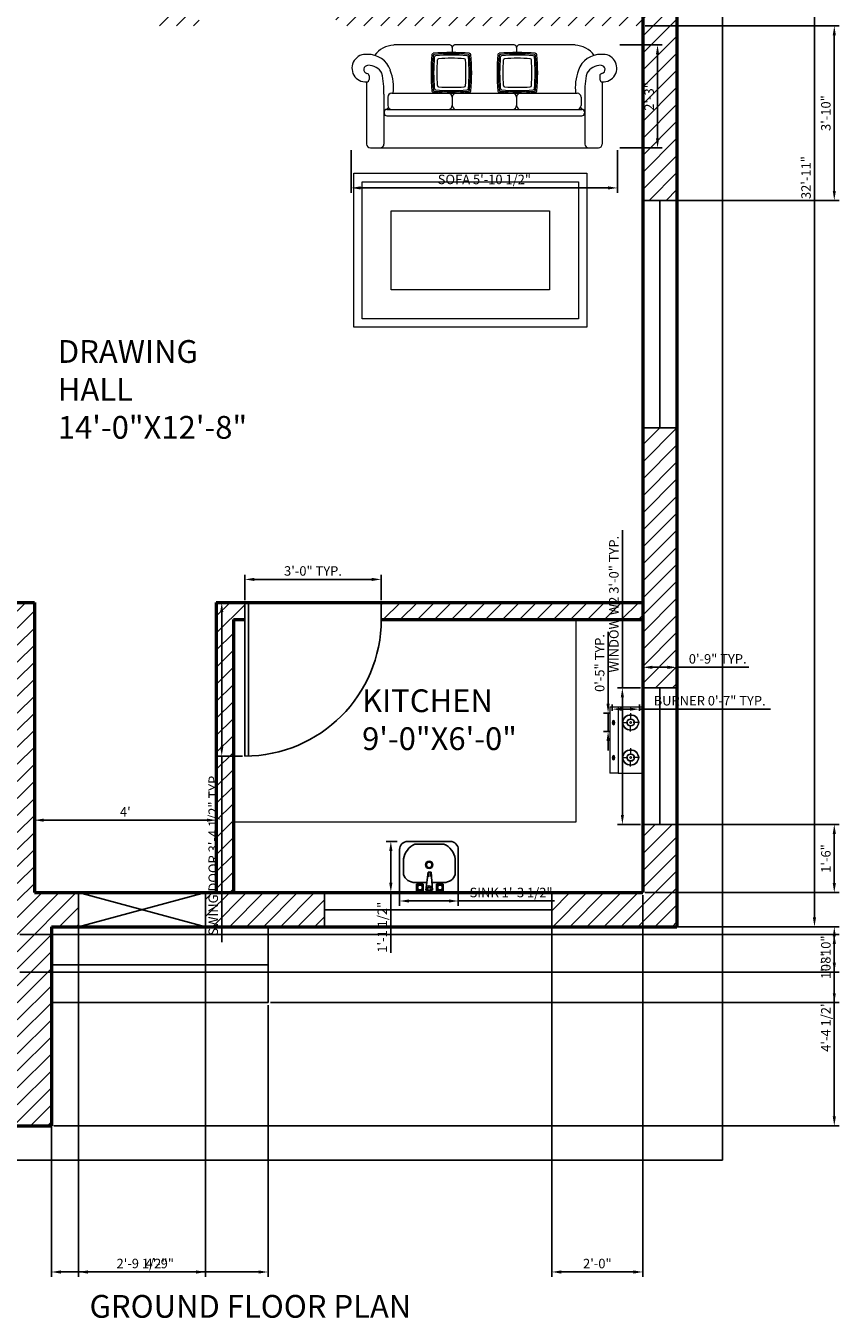
# Model space of a CAD drawing. Units: inches. Extents: x 3542 to 3908, y 2103 to 2666.
# Tile 2 of 4: x 3693 to 3908, y 2103 to 2444. Entities that reach past the tile are written whole.
import ezdxf

# ---------------------------------------------------------------- set-up
doc = ezdxf.new("R2010")
doc.units = ezdxf.units.IN
for name, color, linetype, lineweight in [('A-ANNO-DIMS', 2, 'Continuous', 18), ('A-ANNO-TEXT', 7, 'Continuous', 25), ('A-AREA-IDEN', 7, 'Continuous', 25), ('A-DOOR', 3, 'Continuous', 25), ('A-EQPM', 8, 'Continuous', 18), ('A-FLOR-CASE', 8, 'Continuous', 18), ('A-FLOR-FIXT', 9, 'Continuous', 25), ('A-FLOR-STRS', 7, 'Continuous', 25), ('A-FURN', 8, 'Continuous', 18), ('A-GLAZ', 5, 'Continuous', 25), ('A-WALL', 7, 'Continuous', 50), ('A-WALL-PATT', 252, 'Continuous', 13), ('C-PROP', 7, 'Continuous', 25)]:
    doc.layers.add(name, color=color, linetype=linetype, lineweight=lineweight)
doc.styles.get("Standard").update_dxf_attribs({"font": 'arial.ttf'})
doc.dimstyles.new('ISO-25', dxfattribs={"dimtxt": 2.5, "dimasz": 2.5, "dimexe": 1.25, "dimexo": 0.625, "dimtad": 1, "dimdec": 0, "dimlunit": 3, "dimtxsty": 'Standard', "dimcen": 2.5, "dimadec": 0, "dimazin": 0, "dimtfac": 1, "dimtdec": 0, "dimtmove": 0, "dimatfit": 3, "dimfxl": 1, "dimarcsym": 0})

# ---------------------------------------------------------------- blocks, each defined once
blk = doc.blocks.new('*D1')
at = {"layer": 'A-ANNO-DIMS', "color": 0, "lineweight": -2, "transparency": 16777216}
for p, q in [((3695.14, 2225.85), (3695.14, 2235.83)), ((3743.14, 2225.85), (3743.14, 2235.83)), ((3740.64, 2234.58), (3697.64, 2234.58))]:
    blk.add_line(p, q, dxfattribs=at)
at = {"layer": 'A-ANNO-DIMS', "color": 0, "transparency": 16777216}
for points in [[(3697.64, 2235), (3697.64, 2234.17), (3695.14, 2234.58)], [(3740.64, 2235), (3740.64, 2234.17), (3743.14, 2234.58)]]:
    blk.add_solid(points, dxfattribs=at)
at = {"layer": 'Defpoints', "color": 0, "transparency": 16777216}
for p in [(3695.14, 2234.58), (3695.14, 2225.23), (3743.14, 2225.23)]:
    blk.add_point(p, dxfattribs=at)
at = {"layer": 'A-ANNO-DIMS', "color": 0, "transparency": 16777216, "insert": (3719.14, 2236.46), "char_height": 2.5, "attachment_point": 5}
blk.add_mtext("4'", dxfattribs=at)
blk = doc.blocks.new('*D11')
at = {"layer": 'A-ANNO-DIMS', "color": 0, "lineweight": -2, "transparency": 16777216}
for p, q in [((3877.27, 2601.48), (3902.16, 2601.48)), ((3900.91, 2208.98), (3900.91, 2598.98)), ((3877.27, 2206.48), (3902.16, 2206.48))]:
    blk.add_line(p, q, dxfattribs=at)
at = {"layer": 'A-ANNO-DIMS', "color": 0, "transparency": 16777216}
for points in [[(3900.5, 2598.98), (3901.33, 2598.98), (3900.91, 2601.48)], [(3900.5, 2208.98), (3901.33, 2208.98), (3900.91, 2206.48)]]:
    blk.add_solid(points, dxfattribs=at)
at = {"layer": 'Defpoints', "color": 0, "transparency": 16777216}
for p in [(3876.64, 2601.48), (3900.91, 2601.48), (3876.64, 2206.48)]:
    blk.add_point(p, dxfattribs=at)
at = {"layer": 'A-ANNO-DIMS', "color": 0, "transparency": 16777216, "insert": (3899.01, 2403.98), "char_height": 2.5, "attachment_point": 5, "rotation": 90}
blk.add_mtext('32\'-11"', dxfattribs=at)
blk = doc.blocks.new('A$C796C3687')
for p, q in [((760, 800), (324, 800)), ((760, 800), (324, 800)), ((779, 780), (779, 742)), ((779, 780), (779, 742)), ((1260, 800), (797, 800)), ((1260, 800), (797, 800)), ((1279, 780), (1279, 742)), ((1279, 780), (1279, 742)), ((1734, 800), (1297, 800)), ((1734, 800), (1297, 800)), ((113, 513), (113, 30)), ((113, 513), (113, 30)), ((132, 560), (132, 533)), ((132, 560), (132, 533)), ((1926, 560), (1926, 533)), ((1926, 560), (1926, 533)), ((1945, 513), (1945, 30)), ((1945, 513), (1945, 30)), ((248, 418), (248, 30)), ((248, 418), (248, 30)), ((308, 425), (749, 425)), ((308, 425), (749, 425)), ((809, 425), (1249, 425)), ((809, 425), (1249, 425)), ((1309, 425), (1750, 425)), ((1309, 425), (1750, 425)), ((1810, 418), (1810, 30)), ((1810, 418), (1810, 30)), ((278, 395), (278, 330)), ((278, 395), (278, 330)), ((779, 395), (779, 330)), ((779, 395), (779, 330)), ((1279, 395), (1279, 330)), ((1279, 395), (1279, 330)), ((1780, 395), (1780, 330)), ((1780, 395), (1780, 330)), ((250, 280), (250, 270)), ((250, 280), (250, 270)), ((270, 300), (1787, 300)), ((270, 300), (1787, 300)), ((270, 250), (1787, 250)), ((270, 250), (1787, 250)), ((1807, 280), (1807, 270)), ((1807, 280), (1807, 270)), ((143, 0), (1915, 0)), ((143, 0), (1915, 0))]:
    blk.add_line(p, q)
for centre, radius, start, end in [((106, 620), 107, 83.1024, 273.7108), ((106, 620), 107, 83.1024, 273.7108), ((128, 547), 179, 18.5515, 93.0451), ((128, 547), 179, 18.5515, 93.0451), ((338, 593), 207, 94.0017, 142.3205), ((338, 593), 207, 94.0017, 142.3205), ((2093, 584), 1479, 174.4972, 185.5028), ((2093, 584), 1479, 174.4972, 185.5028), ((631, 725), 10, 95.5028, 174.4972), ((631, 725), 10, 95.5028, 174.4972), ((2093, 584), 1469, 174.8217, 185.1783), ((2093, 584), 1469, 174.8217, 185.1783), ((772, -737), 1479, 84.4972, 95.5028), ((772, -737), 1479, 84.4972, 95.5028), ((640, 716), 10, 95.1783, 174.8217), ((640, 716), 10, 95.1783, 174.8217), ((2093, 584), 1459, 175.1522, 184.8478), ((2093, 584), 1459, 175.1522, 184.8478), ((772, -737), 1469, 84.8217, 95.1783), ((772, -737), 1469, 84.8217, 95.1783), ((650, 706), 10, 94.8478, 175.1522), ((650, 706), 10, 94.8478, 175.1522), ((772, -737), 1459, 85.1522, 94.8478), ((772, -737), 1459, 85.1522, 94.8478), ((759, 780), 20, 0, 94.3856), ((759, 780), 20, 0, 94.3856), ((799, 780), 20, 85.6144, 180), ((799, 780), 20, 85.6144, 180), ((895, 706), 10, 4.8478, 85.1522), ((895, 706), 10, 4.8478, 85.1522), ((904, 716), 10, 5.1783, 84.8217), ((904, 716), 10, 5.1783, 84.8217), ((-549, 584), 1459, 355.1522, 4.8478), ((-549, 584), 1459, 355.1522, 4.8478), ((913, 725), 10, 5.5028, 84.4972), ((913, 725), 10, 5.5028, 84.4972), ((-549, 584), 1469, 354.8217, 5.1783), ((-549, 584), 1469, 354.8217, 5.1783), ((-549, 584), 1479, 354.4972, 5.5028), ((-549, 584), 1479, 354.4972, 5.5028), ((2606, 584), 1479, 174.4972, 185.5028), ((2606, 584), 1479, 174.4972, 185.5028), ((1144, 725), 10, 95.5028, 174.4972), ((1144, 725), 10, 95.5028, 174.4972), ((2606, 584), 1469, 174.8217, 185.1783), ((2606, 584), 1469, 174.8217, 185.1783), ((1285, -737), 1479, 84.4972, 95.5028), ((1285, -737), 1479, 84.4972, 95.5028), ((1154, 716), 10, 95.1783, 174.8217), ((1154, 716), 10, 95.1783, 174.8217), ((2606, 584), 1459, 175.1522, 184.8478), ((2606, 584), 1459, 175.1522, 184.8478), ((1285, -737), 1469, 84.8217, 95.1783), ((1285, -737), 1469, 84.8217, 95.1783), ((1163, 706), 10, 94.8478, 175.1522), ((1163, 706), 10, 94.8478, 175.1522), ((1285, -737), 1459, 85.1522, 94.8478), ((1285, -737), 1459, 85.1522, 94.8478), ((1259, 780), 20, 0, 94.3856), ((1259, 780), 20, 0, 94.3856), ((1299, 780), 20, 85.6144, 180), ((1299, 780), 20, 85.6144, 180), ((1408, 706), 10, 4.8478, 85.1522), ((1408, 706), 10, 4.8478, 85.1522), ((1417, 716), 10, 5.1783, 84.8217), ((1417, 716), 10, 5.1783, 84.8217), ((-36, 584), 1459, 355.1522, 4.8478), ((-36, 584), 1459, 355.1522, 4.8478), ((1426, 725), 10, 5.5028, 84.4972), ((1426, 725), 10, 5.5028, 84.4972), ((-36, 584), 1469, 354.8217, 5.1783), ((-36, 584), 1469, 354.8217, 5.1783), ((-36, 584), 1479, 354.4972, 5.5028), ((-36, 584), 1479, 354.4972, 5.5028), ((1719, 593), 207, 37.6795, 85.9983), ((1719, 593), 207, 37.6795, 85.9983), ((1929, 547), 179, 86.9549, 161.4485), ((1929, 547), 179, 86.9549, 161.4485), ((1951, 620), 107, 266.2892, 96.8976), ((1951, 620), 107, 266.2892, 96.8976), ((122, 610), 31.2, 88.5716, 258.3882), ((122, 610), 31.2, 88.5716, 258.3882), ((126, 520), 122, 29.5431, 91.582), ((126, 520), 122, 29.5431, 91.582), ((-50, 470), 372, 353.0593, 21.0381), ((-50, 470), 372, 353.0593, 21.0381), ((2093, 584), 1434, 176.0063, 183.9937), ((2093, 584), 1434, 176.0063, 183.9937), ((673, 683), 10, 93.9937, 176.0063), ((673, 683), 10, 93.9937, 176.0063), ((772, -737), 1434, 86.0063, 93.9937), ((772, -737), 1434, 86.0063, 93.9937), ((871, 683), 10, 3.9937, 86.0063), ((871, 683), 10, 3.9937, 86.0063), ((-549, 584), 1434, 356.0063, 3.9937), ((-549, 584), 1434, 356.0063, 3.9937), ((2606, 584), 1434, 176.0063, 183.9937), ((2606, 584), 1434, 176.0063, 183.9937), ((1186, 683), 10, 93.9937, 176.0063), ((1186, 683), 10, 93.9937, 176.0063), ((1285, -737), 1434, 86.0063, 93.9937), ((1285, -737), 1434, 86.0063, 93.9937), ((1384, 683), 10, 3.9937, 86.0063), ((1384, 683), 10, 3.9937, 86.0063), ((-36, 584), 1434, 356.0063, 3.9937), ((-36, 584), 1434, 356.0063, 3.9937), ((2107, 470), 372, 158.9619, 187.3268), ((2107, 470), 372, 158.9619, 187.3268), ((1932, 520), 122, 88.418, 150.4569), ((1932, 520), 122, 88.418, 150.4569), ((1936, 610), 31.2, 281.6118, 91.4284), ((1936, 610), 31.2, 281.6118, 91.4284), ((112, 533), 20, 273.7108, 0), ((112, 533), 20, 273.7108, 0), ((112, 560), 20, 0, 78.8393), ((112, 560), 20, 0, 78.8393), ((-351, 440), 599, 357.8297, 13.4516), ((-351, 440), 599, 357.8297, 13.4516), ((2408, 440), 599, 166.5484, 182.1703), ((2408, 440), 599, 166.5484, 182.1703), ((1946, 560), 20, 101.1607, 180), ((1946, 560), 20, 101.1607, 180), ((1946, 533), 20, 180, 266.2892), ((1946, 533), 20, 180, 266.2892), ((308, 395), 30, 90, 180), ((308, 395), 30, 90, 180), ((631, 443), 10, 185.5028, 264.4972), ((631, 443), 10, 185.5028, 264.4972), ((772, 1905), 1479, 264.4972, 275.5028), ((772, 1905), 1479, 264.4972, 275.5028), ((640, 452), 10, 185.1783, 264.8217), ((640, 452), 10, 185.1783, 264.8217), ((650, 462), 10, 184.8478, 265.1522), ((650, 462), 10, 184.8478, 265.1522), ((772, 1905), 1469, 264.8217, 275.1783), ((772, 1905), 1469, 264.8217, 275.1783), ((772, 1905), 1459, 265.1522, 274.8478), ((772, 1905), 1459, 265.1522, 274.8478), ((673, 485), 10, 183.9937, 266.0063), ((673, 485), 10, 183.9937, 266.0063), ((772, 1905), 1434, 266.0063, 273.9937), ((772, 1905), 1434, 266.0063, 273.9937), ((749, 395), 30, 0, 90), ((749, 395), 30, 0, 90), ((809, 395), 30, 90, 180), ((809, 395), 30, 90, 180), ((871, 485), 10, 273.9937, 356.0063), ((871, 485), 10, 273.9937, 356.0063), ((895, 462), 10, 274.8478, 355.1522), ((895, 462), 10, 274.8478, 355.1522), ((904, 452), 10, 275.1783, 354.8217), ((904, 452), 10, 275.1783, 354.8217), ((913, 443), 10, 275.5028, 354.4972), ((913, 443), 10, 275.5028, 354.4972), ((1144, 443), 10, 185.5028, 264.4972), ((1144, 443), 10, 185.5028, 264.4972), ((1285, 1905), 1479, 264.4972, 275.5028), ((1285, 1905), 1479, 264.4972, 275.5028), ((1154, 452), 10, 185.1783, 264.8217), ((1154, 452), 10, 185.1783, 264.8217), ((1163, 462), 10, 184.8478, 265.1522), ((1163, 462), 10, 184.8478, 265.1522), ((1285, 1905), 1469, 264.8217, 275.1783), ((1285, 1905), 1469, 264.8217, 275.1783), ((1285, 1905), 1459, 265.1522, 274.8478), ((1285, 1905), 1459, 265.1522, 274.8478), ((1186, 485), 10, 183.9937, 266.0063), ((1186, 485), 10, 183.9937, 266.0063), ((1285, 1905), 1434, 266.0063, 273.9937), ((1285, 1905), 1434, 266.0063, 273.9937), ((1249, 395), 30, 0, 90), ((1249, 395), 30, 0, 90), ((1309, 395), 30, 90, 180), ((1309, 395), 30, 90, 180), ((1384, 485), 10, 273.9937, 356.0063), ((1384, 485), 10, 273.9937, 356.0063), ((1408, 462), 10, 274.8478, 355.1522), ((1408, 462), 10, 274.8478, 355.1522), ((1417, 452), 10, 275.1783, 354.8217), ((1417, 452), 10, 275.1783, 354.8217), ((1426, 443), 10, 275.5028, 354.4972), ((1426, 443), 10, 275.5028, 354.4972), ((1750, 395), 30, 0, 90), ((1750, 395), 30, 0, 90), ((245, 338), 43.6, 273.0261, 327.6403), ((245, 338), 43.6, 273.0261, 327.6403), ((308, 330), 30, 180, 270), ((308, 330), 30, 180, 270), ((749, 330), 30, 270, 0), ((749, 330), 30, 270, 0), ((809, 330), 30, 180, 270), ((809, 330), 30, 180, 270), ((1249, 330), 30, 270, 0), ((1249, 330), 30, 270, 0), ((1309, 330), 30, 180, 270), ((1309, 330), 30, 180, 270), ((1750, 330), 30, 270, 0), ((1750, 330), 30, 270, 0), ((1812, 338), 43.6, 212.3597, 266.9739), ((1812, 338), 43.6, 212.3597, 266.9739), ((270, 280), 20, 90, 180), ((270, 280), 20, 90, 180), ((270, 270), 20, 180, 270), ((270, 270), 20, 180, 270), ((1787, 280), 20, 0, 90), ((1787, 280), 20, 0, 90), ((1787, 270), 20, 270, 0), ((1787, 270), 20, 270, 0), ((143, 30), 30, 180, 270), ((143, 30), 30, 180, 270), ((218, 30), 30, 270, 0), ((218, 30), 30, 270, 0), ((1840, 30), 30, 180, 270), ((1840, 30), 30, 180, 270), ((1915, 30), 30, 270, 0), ((1915, 30), 30, 270, 0)]:
    blk.add_arc(centre, radius, start, end)
blk = doc.blocks.new('A$C3A735CB7')
for p, q in [((0, 0.38), (0, 0.06)), ((0, 0.38), (0.44, 0.38)), ((0.1148, 0.3068), (0.2035, 0.3068)), ((0.1776, 0.3701), (0.1276, 0.3701)), ((0.1276, 0.3701), (0.1276, 0.3201)), ((0.1276, 0.3201), (0.1776, 0.3201)), ((0.1776, 0.3201), (0.1776, 0.3701)), ((0.1967, 0.364), (0.2114, 0.353)), ((0.2127, 0.229), (0.1967, 0.364)), ((0.1973, 0.3646), (0.2473, 0.3646)), ((0.2114, 0.353), (0.2127, 0.3309)), ((0.247, 0.364), (0.2311, 0.353)), ((0.2311, 0.353), (0.2311, 0.3321)), ((0.2473, 0.3646), (0.236, 0.2302)), ((0.2425, 0.3068), (0.3319, 0.3068)), ((0.2776, 0.3701), (0.2776, 0.3201)), ((0.3276, 0.3701), (0.2776, 0.3701)), ((0.2776, 0.3201), (0.3276, 0.3201)), ((0.3276, 0.3201), (0.3276, 0.3701)), ((0.44, 0.06), (0.44, 0.38)), ((0.0298, 0.1297), (0.0298, 0.2468)), ((0.2114, 0.229), (0.2163, 0.2339)), ((0.236, 0.2302), (0.2127, 0.229)), ((0.2163, 0.2339), (0.2163, 0.2646)), ((0.2323, 0.2327), (0.2323, 0.2634)), ((0.2348, 0.229), (0.2323, 0.2327)), ((0.4169, 0.2468), (0.4169, 0.1297)), ((0.3319, 0.0197), (0.1148, 0.0197)), ((0.06, 0), (0.38, 0))]:
    blk.add_line(p, q)
for centre, radius in [((0.1526, 0.3451), 0.025), ((0.1526, 0.3451), 0.018), ((0.2213, 0.3407), 0.00737), ((0.3026, 0.3451), 0.025), ((0.3026, 0.3451), 0.018), ((0.2215, 0.1752), 0.0272), ((0.2215, 0.1752), 0.0211)]:
    blk.add_circle(centre, radius)
for centre, radius, start, end in [((0.1116, 0.2211), 0.0858, 87.8863, 162.54889), ((0.3351, 0.2211), 0.0858, 17.45111, 92.1137), ((0.1741, 0.1534), 0.1462, 189.3166, 246.07188), ((0.2726, 0.1534), 0.1462, 293.92812, 350.6834), ((0.06, 0.06), 0.06, 180, 270), ((0.38, 0.06), 0.06, 270, 0)]:
    blk.add_arc(centre, radius, start, end)
blk = doc.blocks.new('DOOR-SWING-36IN')
for p, q in [((35, 0), (35, 40.5)), ((36, 4.5), (36, 40.5))]:
    blk.add_line(p, q)
blk.add_arc((36, 4.5), 36, 90, 180)
blk = doc.blocks.new('WIN-60IN')
for p, q in [((0, 60), (0, 0)), ((4.5, 60), (4.5, 0)), ((9, 0), (9, 60))]:
    blk.add_line(p, q)
blk = doc.blocks.new('WIN-36IN')
for p, q in [((0, 36), (0, 0)), ((4.5, 36), (4.5, 0)), ((9, 0), (9, 36))]:
    blk.add_line(p, q)
blk = doc.blocks.new('COOKTOP-BURNER')
for p, q in [((4.84, 4.79), (4.84, 3.05)), ((2.58, 2.36), (4.13, 2.36)), ((4.84, 0), (4.84, 1.68)), ((7.14, 2.33), (5.53, 2.33))]:
    blk.add_line(p, q)
for radius in [2.08, 1.98, 0.995, 0.886, 0.233]:
    blk.add_circle((4.85, 2.34), radius)
at = {"extrusion": (0, 0, -1)}
blk.add_ellipse((0.36, 2.3), major_axis=(0, -0.56), ratio=0.638034, start_param=3.141593, end_param=9.424778, dxfattribs=at)
blk.add_ellipse((0.22, 2.3), major_axis=(0, 0.528), ratio=0.352469, dxfattribs=at)
blk = doc.blocks.new('*D28')
at = {"layer": 'A-ANNO-DIMS', "color": 0, "lineweight": -2, "transparency": 16777216}
for p, q in [((3750.02, 2291.98), (3743.32, 2291.98)), ((3744.57, 2289.48), (3744.57, 2253.98)), ((3750.02, 2251.48), (3743.32, 2251.48)), ((3744.57, 2251.48), (3744.57, 2202.42))]:
    blk.add_line(p, q, dxfattribs=at)
at = {"layer": 'A-ANNO-DIMS', "color": 0, "transparency": 16777216}
for points in [[(3744.15, 2289.48), (3744.99, 2289.48), (3744.57, 2291.98)], [(3744.15, 2253.98), (3744.99, 2253.98), (3744.57, 2251.48)]]:
    blk.add_solid(points, dxfattribs=at)
at = {"layer": 'Defpoints', "color": 0, "transparency": 16777216}
for p in [(3750.64, 2291.98), (3744.57, 2251.48), (3750.64, 2251.48)]:
    blk.add_point(p, dxfattribs=at)
at = {"layer": 'A-ANNO-DIMS', "color": 0, "transparency": 16777216, "insert": (3742.65, 2225.7), "char_height": 2.5, "attachment_point": 5, "rotation": 90}
blk.add_mtext('SWING DOOR 3\'-4 1/2" TYP.', dxfattribs=at)
blk = doc.blocks.new('*D29')
at = {"layer": 'A-ANNO-DIMS', "color": 0, "lineweight": -2, "transparency": 16777216}
for p, q in [((3750.64, 2292.6), (3750.64, 2299.3)), ((3784.14, 2298.05), (3753.14, 2298.05)), ((3786.64, 2292.6), (3786.64, 2299.3))]:
    blk.add_line(p, q, dxfattribs=at)
at = {"layer": 'A-ANNO-DIMS', "color": 0, "transparency": 16777216}
for points in [[(3753.14, 2298.47), (3753.14, 2297.64), (3750.64, 2298.05)], [(3784.14, 2298.47), (3784.14, 2297.64), (3786.64, 2298.05)]]:
    blk.add_solid(points, dxfattribs=at)
at = {"layer": 'Defpoints', "color": 0, "transparency": 16777216}
for p in [(3750.64, 2298.05), (3750.64, 2291.98), (3786.64, 2291.98)]:
    blk.add_point(p, dxfattribs=at)
at = {"layer": 'A-ANNO-DIMS', "color": 0, "transparency": 16777216, "insert": (3768.64, 2299.96), "char_height": 2.5, "attachment_point": 5}
blk.add_mtext('3\'-0" TYP.', dxfattribs=at)
blk = doc.blocks.new('*D32')
at = {"layer": 'A-ANNO-DIMS', "color": 0, "lineweight": -2, "transparency": 16777216}
for p, q in [((3850.24, 2269.48), (3850.24, 2311.07)), ((3855.02, 2269.48), (3848.99, 2269.48)), ((3850.24, 2235.98), (3850.24, 2266.98)), ((3855.02, 2233.48), (3848.99, 2233.48))]:
    blk.add_line(p, q, dxfattribs=at)
at = {"layer": 'A-ANNO-DIMS', "color": 0, "transparency": 16777216}
for points in [[(3849.83, 2266.98), (3850.66, 2266.98), (3850.24, 2269.48)], [(3849.83, 2235.98), (3850.66, 2235.98), (3850.24, 2233.48)]]:
    blk.add_solid(points, dxfattribs=at)
at = {"layer": 'Defpoints', "color": 0, "transparency": 16777216}
for p in [(3850.24, 2269.48), (3855.64, 2269.48), (3855.64, 2233.48)]:
    blk.add_point(p, dxfattribs=at)
at = {"layer": 'A-ANNO-DIMS', "color": 0, "transparency": 16777216, "insert": (3848.33, 2291.53), "char_height": 2.5, "attachment_point": 5, "rotation": 90}
blk.add_mtext('WINDOW W2 3\'-0" TYP.', dxfattribs=at)
blk = doc.blocks.new('*D33')
at = {"layer": 'A-ANNO-DIMS', "color": 0, "lineweight": -2, "transparency": 16777216}
for p, q in [((3855.64, 2270.1), (3855.64, 2276.13)), ((3864.64, 2270.1), (3864.64, 2276.13)), ((3858.14, 2274.88), (3862.14, 2274.88)), ((3864.64, 2274.88), (3883.63, 2274.88))]:
    blk.add_line(p, q, dxfattribs=at)
at = {"layer": 'A-ANNO-DIMS', "color": 0, "transparency": 16777216}
for points in [[(3858.14, 2275.3), (3858.14, 2274.46), (3855.64, 2274.88)], [(3862.14, 2275.3), (3862.14, 2274.46), (3864.64, 2274.88)]]:
    blk.add_solid(points, dxfattribs=at)
at = {"layer": 'Defpoints', "color": 0, "transparency": 16777216}
for p in [(3864.64, 2274.88), (3855.64, 2269.48), (3864.64, 2269.48)]:
    blk.add_point(p, dxfattribs=at)
at = {"layer": 'A-ANNO-DIMS', "color": 0, "transparency": 16777216, "insert": (3875.39, 2276.78), "char_height": 2.5, "attachment_point": 5}
blk.add_mtext('0\'-9" TYP.', dxfattribs=at)
blk = doc.blocks.new('*D40')
at = {"layer": 'A-ANNO-DIMS', "color": 0, "lineweight": -2, "transparency": 16777216}
for p, q in [((3847.55, 2263.4), (3847.55, 2265.1)), ((3850.05, 2263.85), (3852.22, 2263.85)), ((3854.72, 2263.4), (3854.72, 2265.1)), ((3854.72, 2263.85), (3889.32, 2263.85))]:
    blk.add_line(p, q, dxfattribs=at)
at = {"layer": 'A-ANNO-DIMS', "color": 0, "transparency": 16777216}
for points in [[(3850.05, 2264.27), (3850.05, 2263.43), (3847.55, 2263.85)], [(3852.22, 2264.27), (3852.22, 2263.43), (3854.72, 2263.85)]]:
    blk.add_solid(points, dxfattribs=at)
at = {"layer": 'Defpoints', "color": 0, "transparency": 16777216}
for p in [(3847.55, 2262.78), (3854.72, 2263.85), (3854.72, 2262.78)]:
    blk.add_point(p, dxfattribs=at)
at = {"layer": 'A-ANNO-DIMS', "color": 0, "transparency": 16777216, "insert": (3873.27, 2265.75), "char_height": 2.5, "attachment_point": 5}
blk.add_mtext('BURNER 0\'-7" TYP.', dxfattribs=at)
blk = doc.blocks.new('*D41')
at = {"layer": 'A-ANNO-DIMS', "color": 0, "lineweight": -2, "transparency": 16777216}
for p, q in [((3846.48, 2265.28), (3846.48, 2284.26)), ((3846.93, 2262.78), (3845.23, 2262.78)), ((3846.48, 2257.99), (3846.48, 2262.78)), ((3846.93, 2257.99), (3845.23, 2257.99)), ((3846.48, 2255.49), (3846.48, 2252.99))]:
    blk.add_line(p, q, dxfattribs=at)
at = {"layer": 'A-ANNO-DIMS', "color": 0, "transparency": 16777216}
for points in [[(3846.06, 2265.28), (3846.89, 2265.28), (3846.48, 2262.78)], [(3846.06, 2255.49), (3846.89, 2255.49), (3846.48, 2257.99)]]:
    blk.add_solid(points, dxfattribs=at)
at = {"layer": 'Defpoints', "color": 0, "transparency": 16777216}
for p in [(3846.48, 2262.78), (3847.55, 2262.78), (3847.55, 2257.99)]:
    blk.add_point(p, dxfattribs=at)
at = {"layer": 'A-ANNO-DIMS', "color": 0, "transparency": 16777216, "insert": (3844.58, 2276.02), "char_height": 2.5, "attachment_point": 5, "rotation": 90}
blk.add_mtext('0\'-5" TYP.', dxfattribs=at)
blk = doc.blocks.new('*D42')
at = {"layer": 'A-ANNO-DIMS', "color": 0, "lineweight": -2, "transparency": 16777216}
for p, q in [((3778.72, 2411.17), (3778.72, 2400)), ((3848.98, 2411.17), (3848.98, 2400)), ((3781.22, 2401.25), (3846.48, 2401.25))]:
    blk.add_line(p, q, dxfattribs=at)
at = {"layer": 'A-ANNO-DIMS', "color": 0, "transparency": 16777216}
for points in [[(3781.22, 2401.67), (3781.22, 2400.84), (3778.72, 2401.25)], [(3846.48, 2401.67), (3846.48, 2400.84), (3848.98, 2401.25)]]:
    blk.add_solid(points, dxfattribs=at)
at = {"layer": 'Defpoints', "color": 0, "transparency": 16777216}
for p in [(3778.72, 2411.79), (3848.98, 2411.79), (3848.98, 2401.25)]:
    blk.add_point(p, dxfattribs=at)
at = {"layer": 'A-ANNO-DIMS', "color": 0, "transparency": 16777216, "insert": (3813.85, 2403.17), "char_height": 2.5, "attachment_point": 5}
blk.add_mtext('SOFA 5\'-10 1/2"', dxfattribs=at)
blk = doc.blocks.new('*D43')
at = {"layer": 'A-ANNO-DIMS', "color": 0, "lineweight": -2, "transparency": 16777216}
for p, q in [((3849.6, 2438.95), (3860.77, 2438.95)), ((3859.52, 2414.29), (3859.52, 2436.45)), ((3849.6, 2411.79), (3860.77, 2411.79))]:
    blk.add_line(p, q, dxfattribs=at)
at = {"layer": 'A-ANNO-DIMS', "color": 0, "transparency": 16777216}
for points in [[(3859.1, 2436.45), (3859.94, 2436.45), (3859.52, 2438.95)], [(3859.1, 2414.29), (3859.94, 2414.29), (3859.52, 2411.79)]]:
    blk.add_solid(points, dxfattribs=at)
at = {"layer": 'Defpoints', "color": 0, "transparency": 16777216}
for p in [(3848.98, 2438.95), (3859.52, 2438.95), (3848.98, 2411.79)]:
    blk.add_point(p, dxfattribs=at)
at = {"layer": 'A-ANNO-DIMS', "color": 0, "transparency": 16777216, "insert": (3857.62, 2425.37), "char_height": 2.5, "attachment_point": 5, "rotation": 90}
blk.add_mtext('2\'-3"', dxfattribs=at)
blk = doc.blocks.new('*D44')
at = {"layer": 'A-ANNO-DIMS', "color": 0, "lineweight": -2, "transparency": 16777216}
for p, q in [((3791.49, 2214.97), (3791.49, 2212.03)), ((3806.97, 2214.97), (3806.97, 2212.03)), ((3793.99, 2213.28), (3804.47, 2213.28)), ((3806.97, 2213.28), (3832.3, 2213.28))]:
    blk.add_line(p, q, dxfattribs=at)
at = {"layer": 'A-ANNO-DIMS', "color": 0, "transparency": 16777216}
for points in [[(3793.99, 2213.69), (3793.99, 2212.86), (3791.49, 2213.28)], [(3804.47, 2213.69), (3804.47, 2212.86), (3806.97, 2213.28)]]:
    blk.add_solid(points, dxfattribs=at)
at = {"layer": 'Defpoints', "color": 0, "transparency": 16777216}
for p in [(3791.49, 2215.6), (3806.97, 2215.6), (3806.97, 2213.28)]:
    blk.add_point(p, dxfattribs=at)
at = {"layer": 'A-ANNO-DIMS', "color": 0, "transparency": 16777216, "insert": (3820.89, 2215.19), "char_height": 2.5, "attachment_point": 5}
blk.add_mtext('SINK 1\'-3 1/2"', dxfattribs=at)
blk = doc.blocks.new('*D45')
at = {"layer": 'A-ANNO-DIMS', "color": 0, "lineweight": -2, "transparency": 16777216}
for p, q in [((3790.87, 2228.97), (3787.92, 2228.97)), ((3789.17, 2226.47), (3789.17, 2218.1)), ((3790.87, 2215.6), (3787.92, 2215.6)), ((3789.17, 2215.6), (3789.17, 2199.61))]:
    blk.add_line(p, q, dxfattribs=at)
at = {"layer": 'A-ANNO-DIMS', "color": 0, "transparency": 16777216}
for points in [[(3788.75, 2226.47), (3789.59, 2226.47), (3789.17, 2228.97)], [(3788.75, 2218.1), (3789.59, 2218.1), (3789.17, 2215.6)]]:
    blk.add_solid(points, dxfattribs=at)
at = {"layer": 'Defpoints', "color": 0, "transparency": 16777216}
for p in [(3791.49, 2228.97), (3789.17, 2215.6), (3791.49, 2215.6)]:
    blk.add_point(p, dxfattribs=at)
at = {"layer": 'A-ANNO-DIMS', "color": 0, "transparency": 16777216, "insert": (3787.25, 2206.36), "char_height": 2.5, "attachment_point": 5, "rotation": 90}
blk.add_mtext('1\'-1 1/2"', dxfattribs=at)
blk = doc.blocks.new('*D49')
at = {"layer": 'A-ANNO-DIMS', "color": 0, "lineweight": -2, "transparency": 16777216}
for p, q in [((3691.27, 2204.48), (3907.39, 2204.48)), ((3906.14, 2196.98), (3906.14, 2201.98)), ((3691.27, 2194.48), (3907.39, 2194.48))]:
    blk.add_line(p, q, dxfattribs=at)
at = {"layer": 'A-ANNO-DIMS', "color": 0, "transparency": 16777216}
for points in [[(3905.73, 2201.98), (3906.56, 2201.98), (3906.14, 2204.48)], [(3905.73, 2196.98), (3906.56, 2196.98), (3906.14, 2194.48)]]:
    blk.add_solid(points, dxfattribs=at)
at = {"layer": 'Defpoints', "color": 0, "transparency": 16777216}
for p in [(3690.64, 2204.48), (3906.14, 2204.48), (3690.64, 2194.48)]:
    blk.add_point(p, dxfattribs=at)
at = {"layer": 'A-ANNO-DIMS', "color": 0, "transparency": 16777216, "insert": (3904.24, 2199.48), "char_height": 2.5, "attachment_point": 5, "rotation": 90}
blk.add_mtext('0\'-10"', dxfattribs=at)
blk = doc.blocks.new('*D53')
at = {"layer": 'A-ANNO-DIMS', "color": 0, "lineweight": -2, "transparency": 16777216}
for p, q in [((3700.27, 2206.48), (3907.39, 2206.48)), ((3906.14, 2156.48), (3906.14, 2203.98)), ((3700.27, 2153.98), (3907.39, 2153.98))]:
    blk.add_line(p, q, dxfattribs=at)
at = {"layer": 'A-ANNO-DIMS', "color": 0, "transparency": 16777216}
for points in [[(3905.73, 2203.98), (3906.56, 2203.98), (3906.14, 2206.48)], [(3905.73, 2156.48), (3906.56, 2156.48), (3906.14, 2153.98)]]:
    blk.add_solid(points, dxfattribs=at)
at = {"layer": 'Defpoints', "color": 0, "transparency": 16777216}
for p in [(3699.64, 2206.48), (3906.14, 2206.48), (3699.64, 2153.98)]:
    blk.add_point(p, dxfattribs=at)
at = {"layer": 'A-ANNO-DIMS', "color": 0, "transparency": 16777216, "insert": (3904.23, 2180.23), "char_height": 2.5, "attachment_point": 5, "rotation": 90}
blk.add_mtext('4\'-4 1/2"', dxfattribs=at)
blk = doc.blocks.new('*D56')
at = {"layer": 'A-ANNO-DIMS', "color": 0, "lineweight": -2, "transparency": 16777216}
for p, q in [((3831.64, 2214.85), (3831.64, 2114.23)), ((3855.64, 2214.85), (3855.64, 2114.23)), ((3853.14, 2115.48), (3834.14, 2115.48))]:
    blk.add_line(p, q, dxfattribs=at)
at = {"layer": 'A-ANNO-DIMS', "color": 0, "transparency": 16777216}
for points in [[(3834.14, 2115.9), (3834.14, 2115.06), (3831.64, 2115.48)], [(3853.14, 2115.9), (3853.14, 2115.06), (3855.64, 2115.48)]]:
    blk.add_solid(points, dxfattribs=at)
at = {"layer": 'Defpoints', "color": 0, "transparency": 16777216}
for p in [(3831.64, 2215.48), (3855.64, 2215.48), (3831.64, 2115.48)]:
    blk.add_point(p, dxfattribs=at)
at = {"layer": 'A-ANNO-DIMS', "color": 0, "transparency": 16777216, "insert": (3843.64, 2117.38), "char_height": 2.5, "attachment_point": 5}
blk.add_mtext('2\'-0"', dxfattribs=at)
blk = doc.blocks.new('*D57')
at = {"layer": 'A-ANNO-DIMS', "color": 0, "lineweight": -2, "transparency": 16777216}
for p, q in [((3856.27, 2233.48), (3907.39, 2233.48)), ((3906.14, 2230.98), (3906.14, 2217.98)), ((3856.27, 2215.48), (3907.39, 2215.48))]:
    blk.add_line(p, q, dxfattribs=at)
at = {"layer": 'A-ANNO-DIMS', "color": 0, "transparency": 16777216}
for points in [[(3905.73, 2230.98), (3906.56, 2230.98), (3906.14, 2233.48)], [(3905.73, 2217.98), (3906.56, 2217.98), (3906.14, 2215.48)]]:
    blk.add_solid(points, dxfattribs=at)
at = {"layer": 'Defpoints', "color": 0, "transparency": 16777216}
for p in [(3855.64, 2233.48), (3855.64, 2215.48), (3906.14, 2215.48)]:
    blk.add_point(p, dxfattribs=at)
at = {"layer": 'A-ANNO-DIMS', "color": 0, "transparency": 16777216, "insert": (3904.24, 2224.48), "char_height": 2.5, "attachment_point": 5, "rotation": 90}
blk.add_mtext('1\'-6"', dxfattribs=at)
blk = doc.blocks.new('*D60')
at = {"layer": 'A-ANNO-DIMS', "color": 0, "lineweight": -2, "transparency": 16777216}
for p, q in [((3856.27, 2443.98), (3907.39, 2443.98)), ((3906.14, 2400.48), (3906.14, 2441.48)), ((3856.27, 2397.98), (3907.39, 2397.98))]:
    blk.add_line(p, q, dxfattribs=at)
at = {"layer": 'A-ANNO-DIMS', "color": 0, "transparency": 16777216}
for points in [[(3905.73, 2441.48), (3906.56, 2441.48), (3906.14, 2443.98)], [(3905.73, 2400.48), (3906.56, 2400.48), (3906.14, 2397.98)]]:
    blk.add_solid(points, dxfattribs=at)
at = {"layer": 'Defpoints', "color": 0, "transparency": 16777216}
for p in [(3855.64, 2443.98), (3906.14, 2443.98), (3855.64, 2397.98)]:
    blk.add_point(p, dxfattribs=at)
at = {"layer": 'A-ANNO-DIMS', "color": 0, "transparency": 16777216, "insert": (3904.24, 2420.98), "char_height": 2.5, "attachment_point": 5, "rotation": 90}
blk.add_mtext('3\'-10"', dxfattribs=at)
blk = doc.blocks.new('*D62')
at = {"layer": 'A-ANNO-DIMS', "color": 0, "lineweight": -2, "transparency": 16777216}
for p, q in [((3706.76, 2214.85), (3706.76, 2114.23)), ((3740.31, 2214.85), (3740.31, 2114.23)), ((3709.26, 2115.48), (3737.81, 2115.48))]:
    blk.add_line(p, q, dxfattribs=at)
at = {"layer": 'A-ANNO-DIMS', "color": 0, "transparency": 16777216}
for points in [[(3709.26, 2115.9), (3709.26, 2115.06), (3706.76, 2115.48)], [(3737.81, 2115.9), (3737.81, 2115.06), (3740.31, 2115.48)]]:
    blk.add_solid(points, dxfattribs=at)
at = {"layer": 'Defpoints', "color": 0, "transparency": 16777216}
for p in [(3706.76, 2215.48), (3740.31, 2215.48), (3740.31, 2115.48)]:
    blk.add_point(p, dxfattribs=at)
at = {"layer": 'A-ANNO-DIMS', "color": 0, "transparency": 16777216, "insert": (3723.53, 2117.4), "char_height": 2.5, "attachment_point": 5}
blk.add_mtext('2\'-9 1/2"', dxfattribs=at)
blk = doc.blocks.new('*D63')
at = {"layer": 'A-ANNO-DIMS', "color": 0, "lineweight": -2, "transparency": 16777216}
for p, q in [((3699.64, 2185.85), (3699.64, 2114.23)), ((3756.78, 2185.85), (3756.78, 2114.23)), ((3702.14, 2115.48), (3754.28, 2115.48))]:
    blk.add_line(p, q, dxfattribs=at)
at = {"layer": 'A-ANNO-DIMS', "color": 0, "transparency": 16777216}
for points in [[(3702.14, 2115.9), (3702.14, 2115.06), (3699.64, 2115.48)], [(3754.28, 2115.9), (3754.28, 2115.06), (3756.78, 2115.48)]]:
    blk.add_solid(points, dxfattribs=at)
at = {"layer": 'Defpoints', "color": 0, "transparency": 16777216}
for p in [(3699.64, 2186.48), (3756.78, 2186.48), (3756.78, 2115.48)]:
    blk.add_point(p, dxfattribs=at)
at = {"layer": 'A-ANNO-DIMS', "color": 0, "transparency": 16777216, "insert": (3728.21, 2117.38), "char_height": 2.5, "attachment_point": 5}
blk.add_mtext('4\'-9"', dxfattribs=at)
blk = doc.blocks.new('*D64')
at = {"layer": 'A-ANNO-DIMS', "color": 0, "lineweight": -2, "transparency": 16777216}
for p, q in [((3757.4, 2206.48), (3907.39, 2206.48)), ((3906.14, 2188.98), (3906.14, 2203.98)), ((3757.4, 2186.48), (3907.39, 2186.48))]:
    blk.add_line(p, q, dxfattribs=at)
at = {"layer": 'A-ANNO-DIMS', "color": 0, "transparency": 16777216}
for points in [[(3905.73, 2203.98), (3906.56, 2203.98), (3906.14, 2206.48)], [(3905.73, 2188.98), (3906.56, 2188.98), (3906.14, 2186.48)]]:
    blk.add_solid(points, dxfattribs=at)
at = {"layer": 'Defpoints', "color": 0, "transparency": 16777216}
for p in [(3756.78, 2206.48), (3906.14, 2206.48), (3756.78, 2186.48)]:
    blk.add_point(p, dxfattribs=at)
at = {"layer": 'A-ANNO-DIMS', "color": 0, "transparency": 16777216, "insert": (3904.24, 2196.48), "char_height": 2.5, "attachment_point": 5, "rotation": 90}
blk.add_mtext('1\'-8"', dxfattribs=at)

msp = doc.modelspace()

# ---------------------------------------------------------------- hatches: boundary and pattern name
at = {"layer": 'A-WALL-PATT'}
h = msp.add_hatch(dxfattribs=at)
h.set_pattern_fill('ANSI31', color=256)
h.paths.add_polyline_path([(3864.64, 2601.48), (3596.14, 2601.48), (3596.14, 2550.48), (3605.14, 2550.48), (3605.14, 2592.48), (3855.64, 2592.48), (3855.64, 2550.48), (3864.64, 2550.48)])
h.paths.add_polyline_path([(3735.64, 2592.48), (3731.14, 2592.48), (3731.14, 2448.48), (3728.14, 2448.48), (3728.14, 2443.98), (3738.64, 2443.98), (3738.64, 2448.48), (3735.64, 2448.48)])
h.paths.add_polyline_path([(3855.64, 2448.48), (3774.64, 2448.48), (3774.64, 2443.98), (3855.64, 2443.98)])
h.paths.add_polyline_path([(3605.14, 2490.48), (3596.14, 2490.48), (3596.14, 2426.98), (3605.14, 2426.98)])
h.paths.add_polyline_path([(3605.14, 2402.98), (3596.14, 2402.98), (3596.14, 2350.98), (3605.14, 2350.98)])
h.paths.add_polyline_path([(3692.14, 2448.48), (3605.14, 2448.48), (3605.14, 2443.98), (3683.14, 2443.98), (3683.14, 2440.98), (3687.64, 2440.98), (3687.64, 2443.98), (3692.14, 2443.98)])
h.paths.add_polyline_path([(3687.64, 2404.98), (3683.14, 2404.98), (3683.14, 2385.98), (3605.14, 2385.98), (3605.14, 2381.48), (3687.64, 2381.48)])
h.paths.add_polyline_path([(3864.64, 2490.48), (3855.64, 2490.48), (3855.64, 2397.98), (3864.64, 2397.98)])
h.paths.add_polyline_path([(3864.64, 2337.98), (3855.64, 2337.98), (3855.64, 2269.48), (3864.64, 2269.48)])
h.paths.add_polyline_path([(3864.64, 2233.48), (3855.64, 2233.48), (3855.64, 2215.48), (3831.64, 2215.48), (3831.64, 2206.48), (3864.64, 2206.48)])
h.paths.add_polyline_path([(3771.64, 2215.48), (3740.31, 2215.48), (3740.31, 2206.48), (3771.64, 2206.48)])
h.paths.add_polyline_path([(3747.64, 2287.48), (3750.64, 2287.48), (3750.64, 2291.98), (3743.14, 2291.98), (3743.14, 2215.48), (3747.64, 2215.48)])
h.paths.add_polyline_path([(3706.76, 2215.48), (3695.14, 2215.48), (3695.14, 2291.98), (3690.64, 2291.98), (3690.64, 2206.48), (3690.64, 2158.48), (3665.89, 2158.48), (3665.89, 2153.98), (3690.64, 2153.98), (3699.64, 2153.98), (3699.64, 2206.48), (3706.76, 2206.48)])
h.paths.add_polyline_path([(3605.14, 2314.98), (3596.14, 2314.98), (3596.14, 2153.98), (3629.89, 2153.98), (3629.89, 2158.48), (3605.14, 2158.48)])
h = msp.add_hatch(dxfattribs=at)
h.set_pattern_fill('ANSI31', color=256)
h.paths.add_polyline_path([(3855.64, 2291.98), (3786.64, 2291.98), (3786.64, 2287.48), (3855.64, 2287.48)])

# ---------------------------------------------------------------- linework, layer by layer
at = {"layer": 'A-DOOR'}
for p, q in [((3750.64, 2287.48), (3750.64, 2291.98)), ((3786.64, 2291.98), (3786.64, 2287.48)), ((3706.76, 2215.48), (3706.76, 2206.48)), ((3740.31, 2215.48), (3706.76, 2215.48)), ((3706.76, 2215.48), (3740.31, 2206.48)), ((3740.31, 2215.48), (3706.76, 2206.48)), ((3740.31, 2206.48), (3740.31, 2215.48)), ((3706.76, 2206.48), (3740.31, 2206.48))]:
    msp.add_line(p, q, dxfattribs=at)
at = {"layer": 'A-EQPM'}
for p, q in [((3846.93, 2264.39), (3846.93, 2246.96)), ((3849.11, 2264.39), (3846.93, 2264.39)), ((3855.64, 2264.39), (3849.11, 2264.39)), ((3849.11, 2264.39), (3849.11, 2246.96)), ((3855.64, 2246.96), (3855.64, 2264.39)), ((3849.11, 2246.96), (3846.93, 2246.96)), ((3849.11, 2246.96), (3855.64, 2246.96))]:
    msp.add_line(p, q, dxfattribs=at)
at = {"layer": 'A-FLOR-CASE'}
for p, q in [((3838.05, 2234.12), (3838.05, 2287.48)), ((3747.64, 2234.12), (3747.64, 2234.12)), ((3747.64, 2234.12), (3838.05, 2234.12))]:
    msp.add_line(p, q, dxfattribs=at)
at = {"layer": 'A-FLOR-STRS'}
for p, q in [((3756.78, 2206.48), (3756.78, 2186.48)), ((3699.64, 2196.48), (3756.78, 2196.48)), ((3699.64, 2186.48), (3756.78, 2186.48))]:
    msp.add_line(p, q, dxfattribs=at)
at = {"layer": 'A-FURN'}
for points in [[(3840.9, 2405.15), (3840.9, 2364.51), (3779.39, 2364.51), (3779.39, 2405.15)], [(3838.65, 2402.9), (3838.65, 2366.76), (3781.65, 2366.76), (3781.65, 2402.9)], [(3838.65, 2402.9), (3838.65, 2366.76), (3781.65, 2366.76), (3781.65, 2402.9)], [(3830.99, 2395.24), (3830.99, 2374.41), (3789.3, 2374.41), (3789.3, 2395.24)]]:
    msp.add_lwpolyline(points, close=True, dxfattribs=at)
at = {"layer": 'A-GLAZ'}
for p, q in [((3864.64, 2397.98), (3855.64, 2397.98)), ((3855.64, 2337.98), (3864.64, 2337.98)), ((3864.64, 2269.48), (3855.64, 2269.48)), ((3855.64, 2233.48), (3864.64, 2233.48)), ((3771.64, 2206.48), (3771.64, 2215.48)), ((3831.64, 2215.48), (3831.64, 2206.48))]:
    msp.add_line(p, q, dxfattribs=at)
at = {"layer": 'A-WALL'}
for p, q in [((3864.64, 2601.48), (3864.64, 2206.48)), ((3855.64, 2592.48), (3855.64, 2215.48)), ((3690.64, 2291.98), (3695.14, 2291.98)), ((3695.14, 2291.98), (3695.14, 2215.48)), ((3743.14, 2291.98), (3743.14, 2215.48)), ((3743.14, 2291.98), (3855.64, 2291.98)), ((3747.64, 2287.48), (3750.64, 2287.48)), ((3747.64, 2287.48), (3747.64, 2215.48)), ((3786.64, 2287.48), (3855.64, 2287.48)), ((3695.14, 2215.48), (3855.64, 2215.48)), ((3699.64, 2206.48), (3864.64, 2206.48)), ((3699.64, 2206.48), (3699.64, 2153.98)), ((3690.64, 2153.98), (3699.64, 2153.98))]:
    msp.add_line(p, q, dxfattribs=at)
at = {"layer": 'C-PROP'}
for p, q in [((3876.64, 2601.48), (3876.64, 2206.48)), ((3864.64, 2206.48), (3876.64, 2206.48)), ((3876.64, 2206.48), (3876.64, 2206.48)), ((3876.64, 2206.48), (3876.64, 2144.98)), ((3690.64, 2144.98), (3864.64, 2144.98)), ((3876.64, 2144.98), (3864.64, 2144.98))]:
    msp.add_line(p, q, dxfattribs=at)

# ---------------------------------------------------------------- block references
at = {"layer": 'A-DOOR', "rotation": 180}
msp.add_blockref('DOOR-SWING-36IN', (3786.64, 2291.98), dxfattribs=at)
at = {"layer": 'A-EQPM'}
for p in [(3847.58, 2257.99), (3847.58, 2248.76)]:
    msp.add_blockref('COOKTOP-BURNER', p, dxfattribs=at)
at = {"layer": 'A-FLOR-FIXT', "xscale": -35.18874060287814, "yscale": 35.18874060287814, "zscale": 35.18874060287814, "rotation": 180}
msp.add_blockref('A$C3A735CB7', (3791.49, 2228.97), dxfattribs=at)
at = {"layer": 'A-FURN', "xscale": 0.0339292347498656, "yscale": 0.0339292347498656, "zscale": 0.0339292347498656}
msp.add_blockref('A$C796C3687', (3778.95, 2411.79), dxfattribs=at)
at = {"layer": 'A-GLAZ'}
for name, p in [('WIN-60IN', (3855.64, 2337.98)), ('WIN-36IN', (3855.64, 2233.48))]:
    msp.add_blockref(name, p, dxfattribs=at)
at = {"layer": 'A-GLAZ', "rotation": 270}
msp.add_blockref('WIN-60IN', (3771.64, 2215.48), dxfattribs=at)

# ---------------------------------------------------------------- texts
at = {"layer": 'A-ANNO-TEXT', "insert": (3709.7, 2109.42), "char_height": 6, "attachment_point": 1}
msp.add_mtext('GROUND FLOOR PLAN', dxfattribs=at)
at = {"layer": 'A-AREA-IDEN', "char_height": 6, "attachment_point": 1}
for s, width, insert in [('DRAWING HALL\\P14\'-0"X12\'-8"', 27.5926, (3701.33, 2361.14)), ('KITCHEN\\P9\'-0"X6\'-0"', 16.5919, (3781.58, 2269.07))]:
    msp.add_mtext_dynamic_manual_height_columns(s, width=width, gutter_width=12.5, heights=[0], dxfattribs=dict(at, insert=insert))

# ---------------------------------------------------------------- dimensions: what is measured, and where the dimension line sits
at = {"layer": 'A-ANNO-DIMS'}
for base, p1, p2, angle, override, picture, middle in [((3900.91, 2601.48), (3876.64, 2206.48), (3876.64, 2601.48), 90, {"dimclrd": 0, "dimclre": 0, "dimclrt": 0}, '*D11', (3899.01, 2403.98)), ((3906.14, 2443.98), (3855.64, 2397.98), (3855.64, 2443.98), 90, {"dimdec": 1, "dimlfac": 1, "dimrnd": 0, "dimzin": 1, "dimdsep": 46, "dimlunit": 4, "dimfrac": 2}, '*D60', (3904.24, 2420.98)), ((3859.52, 2438.95), (3848.98, 2411.79), (3848.98, 2438.95), 90, {"dimdec": 1, "dimlfac": 1, "dimrnd": 0, "dimzin": 1, "dimdsep": 46, "dimlunit": 4, "dimfrac": 2}, '*D43', (3857.62, 2425.37)), ((3906.14, 2215.48), (3855.64, 2233.48), (3855.64, 2215.48), 90, {"dimdec": 1, "dimlfac": 1, "dimrnd": 0, "dimzin": 1, "dimdsep": 46, "dimlunit": 4, "dimfrac": 2}, '*D57', (3904.24, 2224.48)), ((3789.17, 2215.6), (3791.49, 2228.97), (3791.49, 2215.6), 270, {"dimdec": 1, "dimlfac": 1, "dimrnd": 0, "dimzin": 1, "dimdsep": 46, "dimlunit": 4, "dimfrac": 2}, '*D45', (3787.25, 2206.36)), ((3906.14, 2204.48), (3690.64, 2194.48), (3690.64, 2204.48), 90, {"dimdec": 1, "dimlfac": 1, "dimrnd": 0, "dimzin": 1, "dimdsep": 46, "dimlunit": 4, "dimfrac": 2}, '*D49', (3904.24, 2199.48)), ((3906.14, 2206.48), (3699.64, 2153.98), (3699.64, 2206.48), 90, {"dimdec": 1, "dimlfac": 1, "dimrnd": 0, "dimzin": 1, "dimdsep": 46, "dimlunit": 4, "dimfrac": 2}, '*D53', (3904.23, 2180.23)), ((3906.14, 2206.48), (3756.78, 2186.48), (3756.78, 2206.48), 90, {"dimdec": 1, "dimlfac": 1, "dimrnd": 0, "dimzin": 1, "dimdsep": 46, "dimlunit": 4, "dimfrac": 2}, '*D64', (3904.24, 2196.48))]:
    dim = msp.add_linear_dim(base=base, p1=p1, p2=p2, angle=angle, dimstyle='ISO-25', override=override, dxfattribs=at)
    dim.commit()
    dim.dimension.update_dxf_attribs({"geometry": picture, "text_midpoint": middle})
for base, p1, p2, text, picture, middle in [((3848.98, 2401.25), (3778.72, 2411.79), (3848.98, 2411.79), 'SOFA <>', '*D42', (3813.85, 2403.17)), ((3864.64, 2274.88), (3855.64, 2269.48), (3864.64, 2269.48), '<> TYP.', '*D33', (3875.39, 2276.78)), ((3854.72, 2263.85), (3847.55, 2262.78), (3854.72, 2262.78), 'BURNER <> TYP.', '*D40', (3873.27, 2265.75)), ((3806.97, 2213.28), (3791.49, 2215.6), (3806.97, 2215.6), 'SINK <>', '*D44', (3820.89, 2215.19))]:
    dim = msp.add_linear_dim(base=base, p1=p1, p2=p2, text=text, dimstyle='ISO-25', override={"dimdec": 1, "dimlfac": 1, "dimrnd": 0, "dimzin": 1, "dimdsep": 46, "dimlunit": 4, "dimfrac": 2}, dxfattribs=at)
    dim.commit()
    dim.dimension.update_dxf_attribs({"geometry": picture, "text_midpoint": middle})
for base, p1, p2, angle, text, picture, middle in [((3850.24, 2269.48), (3855.64, 2233.48), (3855.64, 2269.48), 90, 'WINDOW W2 <> TYP.', '*D32', (3848.33, 2291.53)), ((3750.64, 2298.05), (3786.64, 2291.98), (3750.64, 2291.98), 180, '<> TYP.', '*D29', (3768.64, 2299.96)), ((3744.57, 2251.48), (3750.64, 2291.98), (3750.64, 2251.48), 270, 'SWING DOOR <> TYP.', '*D28', (3742.65, 2225.7)), ((3846.48, 2262.78), (3847.55, 2257.99), (3847.55, 2262.78), 90, '<> TYP.', '*D41', (3844.58, 2276.02))]:
    dim = msp.add_linear_dim(base=base, p1=p1, p2=p2, angle=angle, text=text, dimstyle='ISO-25', override={"dimdec": 1, "dimlfac": 1, "dimrnd": 0, "dimzin": 1, "dimdsep": 46, "dimlunit": 4, "dimfrac": 2}, dxfattribs=at)
    dim.commit()
    dim.dimension.update_dxf_attribs({"geometry": picture, "text_midpoint": middle})
for base, p1, p2, override, picture, middle in [((3695.14, 2234.58), (3743.14, 2225.23), (3695.14, 2225.23), {"dimclrd": 0, "dimclre": 0, "dimclrt": 0}, '*D1', (3719.14, 2236.46)), ((3740.31, 2115.4792), (3706.7587, 2215.4792), (3740.31, 2215.4792), {"dimdec": 1, "dimlfac": 1, "dimrnd": 0, "dimzin": 1, "dimdsep": 46, "dimlunit": 4, "dimfrac": 2}, '*D62', (3723.5343, 2117.3968)), ((3831.64, 2115.48), (3855.64, 2215.48), (3831.64, 2215.48), {"dimdec": 1, "dimlfac": 1, "dimrnd": 0, "dimzin": 1, "dimdsep": 46, "dimlunit": 4, "dimfrac": 2}, '*D56', (3843.64, 2117.38)), ((3756.78, 2115.48), (3699.64, 2186.48), (3756.78, 2186.48), {"dimdec": 1, "dimlfac": 1, "dimrnd": 0, "dimzin": 1, "dimdsep": 46, "dimlunit": 4, "dimfrac": 2}, '*D63', (3728.21, 2117.38))]:
    dim = msp.add_linear_dim(base=base, p1=p1, p2=p2, dimstyle='ISO-25', override=override, dxfattribs=at)
    dim.commit()
    dim.dimension.update_dxf_attribs({"geometry": picture, "text_midpoint": middle})

doc.saveas('drawing.dxf')
